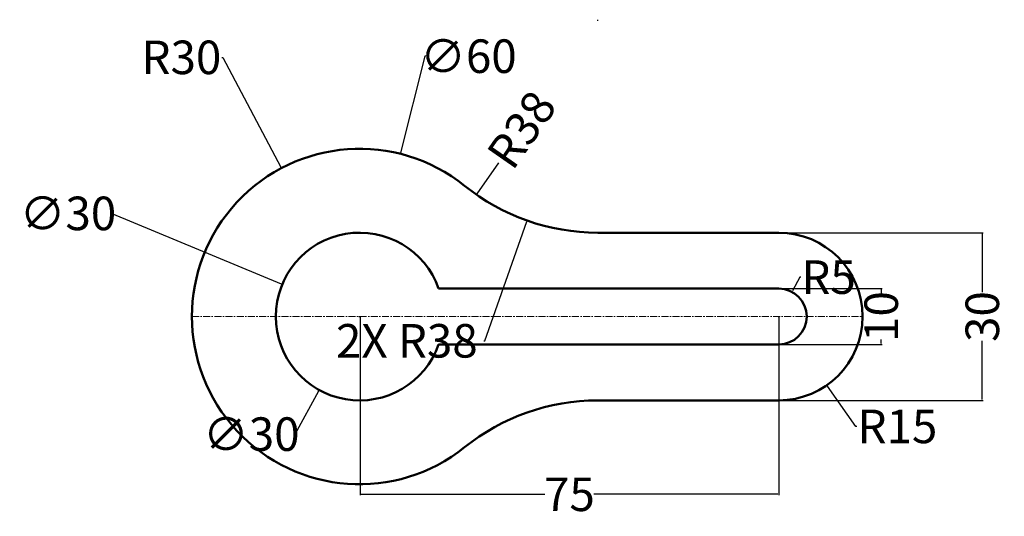
# Model space of a CAD drawing. Units: millimetres. Extents: x 2 to 178, y 21 to 110.
import ezdxf

# ---------------------------------------------------------------- set-up
doc = ezdxf.new("R2010")
doc.units = ezdxf.units.MM
doc.header["$MEASUREMENT"] = 0
doc.linetypes.add('CENTER', pattern=[2, 1.25, -0.25, 0.25, -0.25])
for name, color, linetype, lineweight in [('M-CNTR', 4, 'CENTER', 18), ('M-DIMS', 2, 'Continuous', 25), ('M-OUTL', 7, 'Continuous', 50)]:
    doc.layers.add(name, color=color, linetype=linetype, lineweight=lineweight)
doc.styles.get("Standard").update_dxf_attribs({"font": 'arial.ttf'})
doc.dimstyles.get("Standard").update_dxf_attribs({"dimtxt": 6, "dimasz": 0.18, "dimexe": 0.18, "dimexo": 0.0625, "dimgap": 0.09, "dimtad": 0, "dimtoh": 1, "dimdec": 0, "dimzin": 0, "dimdsep": 46, "dimtxsty": 'Standard', "dimcen": 0.09, "dimadec": 0, "dimazin": 0, "dimtfac": 1, "dimtdec": 0, "dimtofl": 0, "dimtmove": 0, "dimatfit": 3, "dimfxl": 1, "dimtolj": 1, "dimtzin": 0, "dimarcsym": 0})

# ---------------------------------------------------------------- blocks, each defined once
blk = doc.blocks.new('*D1')
at = {"layer": 'Defpoints', "color": 0, "transparency": 16777216}
for p in [(48.73, 83.47), (62.73, 56.94)]:
    blk.add_point(p, dxfattribs=at)
at = {"layer": 'M-DIMS', "color": 0, "lineweight": -2, "transparency": 16777216}
for p, q in [((38.08, 103.3), (38.26, 103.3)), ((38.26, 103.3), (48.64, 83.63)), ((62.64, 56.94), (62.82, 56.94)), ((62.73, 56.85), (62.73, 57.03))]:
    blk.add_line(p, q, dxfattribs=at)
at = {"layer": 'M-DIMS', "color": 0, "transparency": 16777216}
blk.add_solid([(48.67, 83.65), (48.61, 83.62), (48.73, 83.47)], dxfattribs=at)
at = {"layer": 'M-DIMS', "color": 0, "transparency": 16777216, "insert": (30.83, 103.3), "char_height": 6, "attachment_point": 5}
blk.add_mtext('\\A1;R30', dxfattribs=at)
blk = doc.blocks.new('*D2')
at = {"layer": 'Defpoints', "color": 0, "transparency": 16777216}
for p in [(105.33, 109.94), (83.61, 78.76)]:
    blk.add_point(p, dxfattribs=at)
at = {"layer": 'M-DIMS', "color": 0, "lineweight": -2, "transparency": 16777216}
blk.add_line((87.56, 84.43), (83.71, 78.91), dxfattribs=at)
at = {"layer": 'M-DIMS', "color": 0, "transparency": 16777216}
blk.add_solid([(83.69, 78.93), (83.74, 78.89), (83.61, 78.76)], dxfattribs=at)
at = {"layer": 'M-DIMS', "color": 0, "transparency": 16777216, "insert": (91.71, 90.39), "char_height": 6, "attachment_point": 5, "rotation": 55.1393}
blk.add_mtext('\\A1;R38', dxfattribs=at)
blk = doc.blocks.new('*D3')
at = {"layer": 'Defpoints', "color": 0, "transparency": 16777216}
for p in [(62.82, 56.94), (137.73, 56.94), (137.73, 25.15)]:
    blk.add_point(p, dxfattribs=at)
at = {"layer": 'M-DIMS', "color": 0, "lineweight": -2, "transparency": 16777216}
for p, q in [((62.82, 56.88), (62.82, 24.97)), ((137.73, 56.88), (137.73, 24.97)), ((63, 25.15), (95.89, 25.15)), ((137.55, 25.15), (104.66, 25.15))]:
    blk.add_line(p, q, dxfattribs=at)
at = {"layer": 'M-DIMS', "color": 0, "transparency": 16777216}
for points in [[(63, 25.18), (63, 25.12), (62.82, 25.15)], [(137.55, 25.18), (137.55, 25.12), (137.73, 25.15)]]:
    blk.add_solid(points, dxfattribs=at)
at = {"layer": 'M-DIMS', "color": 0, "transparency": 16777216, "insert": (100.27, 25.15), "char_height": 6, "attachment_point": 5}
blk.add_mtext('\\A1;75', dxfattribs=at)
blk = doc.blocks.new('*D4')
at = {"layer": 'Defpoints', "color": 0, "transparency": 16777216}
for p in [(137.73, 71.94), (137.73, 41.94), (174.16, 41.94)]:
    blk.add_point(p, dxfattribs=at)
at = {"layer": 'M-DIMS', "color": 0, "lineweight": -2, "transparency": 16777216}
for p, q in [((137.79, 71.94), (174.34, 71.94)), ((174.16, 71.76), (174.16, 61.32)), ((174.16, 42.12), (174.16, 52.57)), ((137.79, 41.94), (174.34, 41.94))]:
    blk.add_line(p, q, dxfattribs=at)
at = {"layer": 'M-DIMS', "color": 0, "transparency": 16777216}
for points in [[(174.13, 71.76), (174.19, 71.76), (174.16, 71.94)], [(174.13, 42.12), (174.19, 42.12), (174.16, 41.94)]]:
    blk.add_solid(points, dxfattribs=at)
at = {"layer": 'M-DIMS', "color": 0, "transparency": 16777216, "insert": (174.16, 56.94), "char_height": 6, "attachment_point": 5, "rotation": 90}
blk.add_mtext('\\A1;30', dxfattribs=at)
blk = doc.blocks.new('*D5')
at = {"layer": 'Defpoints', "color": 0, "transparency": 16777216}
for p in [(137.73, 61.94), (137.73, 51.94), (156.07, 51.94)]:
    blk.add_point(p, dxfattribs=at)
at = {"layer": 'M-DIMS', "color": 0, "lineweight": -2, "transparency": 16777216}
for p, q in [((137.79, 61.94), (156.25, 61.94)), ((156.07, 61.76), (156.07, 61.04)), ((137.79, 51.94), (156.25, 51.94)), ((156.07, 52.12), (156.07, 52.85))]:
    blk.add_line(p, q, dxfattribs=at)
at = {"layer": 'M-DIMS', "color": 0, "transparency": 16777216}
for points in [[(156.04, 61.76), (156.1, 61.76), (156.07, 61.94)], [(156.04, 52.12), (156.1, 52.12), (156.07, 51.94)]]:
    blk.add_solid(points, dxfattribs=at)
at = {"layer": 'M-DIMS', "color": 0, "transparency": 16777216, "insert": (156.07, 56.94), "char_height": 6, "attachment_point": 5, "rotation": 90}
blk.add_mtext('\\A1;10', dxfattribs=at)
blk = doc.blocks.new('*D6')
at = {"layer": 'Defpoints', "color": 0, "transparency": 16777216}
for p in [(48.88, 62.7), (76.58, 51.19)]:
    blk.add_point(p, dxfattribs=at)
at = {"layer": 'M-DIMS', "color": 0, "lineweight": -2, "transparency": 16777216}
for p, q in [((18.17, 75.39), (18.35, 75.39)), ((18.35, 75.39), (48.71, 62.77)), ((62.64, 56.94), (62.82, 56.94)), ((62.73, 56.85), (62.73, 57.03))]:
    blk.add_line(p, q, dxfattribs=at)
at = {"layer": 'M-DIMS', "color": 0, "transparency": 16777216}
blk.add_solid([(48.72, 62.8), (48.7, 62.74), (48.88, 62.7)], dxfattribs=at)
at = {"layer": 'M-DIMS', "color": 0, "transparency": 16777216, "insert": (10.53, 75.39), "char_height": 6, "attachment_point": 5}
blk.add_mtext('\\A1;∅30', dxfattribs=at)
blk = doc.blocks.new('*D7')
at = {"layer": 'Defpoints', "color": 0, "transparency": 16777216}
for p in [(70.01, 86.05), (55.45, 27.84)]:
    blk.add_point(p, dxfattribs=at)
at = {"layer": 'M-DIMS', "color": 0, "lineweight": -2, "transparency": 16777216}
for p, q in [((74.38, 103.51), (70.06, 86.22)), ((74.56, 103.51), (74.38, 103.51)), ((62.64, 56.94), (62.82, 56.94)), ((62.73, 56.85), (62.73, 57.03))]:
    blk.add_line(p, q, dxfattribs=at)
at = {"layer": 'M-DIMS', "color": 0, "transparency": 16777216}
blk.add_solid([(70.03, 86.23), (70.08, 86.21), (70.01, 86.05)], dxfattribs=at)
at = {"layer": 'M-DIMS', "color": 0, "transparency": 16777216, "insert": (82.2, 103.51), "char_height": 6, "attachment_point": 5}
blk.add_mtext('\\A1;∅60', dxfattribs=at)
blk = doc.blocks.new('*D8')
at = {"layer": 'Defpoints', "color": 0, "transparency": 16777216}
for p in [(69.96, 70.09), (55.5, 43.8)]:
    blk.add_point(p, dxfattribs=at)
at = {"layer": 'M-DIMS', "color": 0, "lineweight": -2, "transparency": 16777216}
for p, q in [((62.64, 56.94), (62.82, 56.94)), ((62.73, 56.85), (62.73, 57.03)), ((51.16, 35.91), (55.41, 43.64)), ((50.98, 35.91), (51.16, 35.91))]:
    blk.add_line(p, q, dxfattribs=at)
at = {"layer": 'M-DIMS', "color": 0, "transparency": 16777216}
blk.add_solid([(55.39, 43.66), (55.44, 43.63), (55.5, 43.8)], dxfattribs=at)
at = {"layer": 'M-DIMS', "color": 0, "transparency": 16777216, "insert": (43.34, 35.91), "char_height": 6, "attachment_point": 5}
blk.add_mtext('\\A1;∅30', dxfattribs=at)
blk = doc.blocks.new('*D9')
at = {"layer": 'Defpoints', "color": 0, "transparency": 16777216}
for p in [(105.33, 109.94), (92.7, 74.1)]:
    blk.add_point(p, dxfattribs=at)
at = {"layer": 'M-DIMS', "color": 0, "lineweight": -2, "transparency": 16777216}
for p, q in [((105.24, 109.94), (105.42, 109.94)), ((105.33, 109.85), (105.33, 110.03)), ((85.12, 52.6), (92.64, 73.93)), ((84.94, 52.6), (85.12, 52.6))]:
    blk.add_line(p, q, dxfattribs=at)
at = {"layer": 'M-DIMS', "color": 0, "transparency": 16777216}
blk.add_solid([(92.61, 73.94), (92.67, 73.92), (92.7, 74.1)], dxfattribs=at)
at = {"layer": 'M-DIMS', "color": 0, "transparency": 16777216, "insert": (71.18, 52.6), "char_height": 6, "attachment_point": 5}
blk.add_mtext('\\A1;2X R38', dxfattribs=at)
blk = doc.blocks.new('*D10')
at = {"layer": 'Defpoints', "color": 0, "transparency": 16777216}
for p in [(137.73, 56.94), (146.34, 44.66)]:
    blk.add_point(p, dxfattribs=at)
at = {"layer": 'M-DIMS', "color": 0, "lineweight": -2, "transparency": 16777216}
for p, q in [((137.64, 56.94), (137.82, 56.94)), ((137.73, 56.85), (137.73, 57.03)), ((151.51, 37.29), (146.44, 44.51)), ((151.69, 37.29), (151.51, 37.29))]:
    blk.add_line(p, q, dxfattribs=at)
at = {"layer": 'M-DIMS', "color": 0, "transparency": 16777216}
blk.add_solid([(146.47, 44.53), (146.42, 44.5), (146.34, 44.66)], dxfattribs=at)
at = {"layer": 'M-DIMS', "color": 0, "transparency": 16777216, "insert": (158.97, 37.29), "char_height": 6, "attachment_point": 5}
blk.add_mtext('\\A1;R15', dxfattribs=at)
blk = doc.blocks.new('*D11')
at = {"layer": 'Defpoints', "color": 0, "transparency": 16777216}
for p in [(140.1, 61.35), (137.73, 56.94)]:
    blk.add_point(p, dxfattribs=at)
at = {"layer": 'M-DIMS', "color": 0, "lineweight": -2, "transparency": 16777216}
for p, q in [((141.52, 63.99), (140.18, 61.51)), ((141.7, 63.99), (141.52, 63.99)), ((137.64, 56.94), (137.82, 56.94)), ((137.73, 56.85), (137.73, 57.03))]:
    blk.add_line(p, q, dxfattribs=at)
at = {"layer": 'M-DIMS', "color": 0, "transparency": 16777216}
blk.add_solid([(140.16, 61.52), (140.21, 61.49), (140.1, 61.35)], dxfattribs=at)
at = {"layer": 'M-DIMS', "color": 0, "transparency": 16777216, "insert": (146.65, 63.99), "char_height": 6, "attachment_point": 5}
blk.add_mtext('\\A1;R5', dxfattribs=at)

msp = doc.modelspace()

# ---------------------------------------------------------------- linework, layer by layer
at = {"layer": 'M-CNTR'}
msp.add_line((32.73, 56.94), (152.73, 56.94), dxfattribs=at)
at = {"layer": 'M-OUTL'}
for points in [[(81.52, 80.33, 0.170903), (105.33, 71.94), (137.73, 71.94, -1), (137.73, 41.94), (105.33, 41.94, 0.170903), (81.52, 33.56, -2.086846)], [(76.87, 61.94), (137.73, 61.94, -1), (137.73, 51.94), (76.87, 51.94, -5.828427)]]:
    msp.add_lwpolyline(points, format="xyb", close=True, dxfattribs=at)

# ---------------------------------------------------------------- dimensions: what is measured, and where the dimension line sits
at = {"layer": 'M-DIMS'}
dim = msp.add_radius_dim(center=(105.33, 109.94), mpoint=(92.7, 74.1), text='2X <>', dimstyle='Standard', override={"dimdec": 0, "dimlfac": 1, "dimrnd": 0, "dimzin": 0, "dimdsep": 46, "dimlunit": 2}, dxfattribs=at)
dim.commit()
dim.dimension.update_dxf_attribs({"geometry": '*D9', "text_midpoint": (71.18, 52.6), "dimtype": 164})
for center, mpoint, override, picture, middle in [((105.33, 109.94), (83.61, 78.76), {"dimclrd": 0, "dimclre": 0, "dimclrt": 0}, '*D2', (91.71, 90.39)), ((62.73, 56.94), (48.73, 83.47), {"dimclrd": 0, "dimclre": 0, "dimclrt": 0}, '*D1', (30.83, 103.3)), ((137.73, 56.94), (140.1, 61.35), {"dimdec": 0, "dimlfac": 1, "dimrnd": 0, "dimzin": 0, "dimdsep": 46, "dimlunit": 2}, '*D11', (146.65, 63.99)), ((137.73, 56.94), (146.34, 44.66), {"dimdec": 0, "dimlfac": 1, "dimrnd": 0, "dimzin": 0, "dimdsep": 46, "dimlunit": 2}, '*D10', (158.97, 37.29))]:
    dim = msp.add_radius_dim(center=center, mpoint=mpoint, dimstyle='Standard', override=override, dxfattribs=at)
    dim.commit()
    dim.dimension.update_dxf_attribs({"geometry": picture, "text_midpoint": middle, "dimtype": 164})
for p1, p2, override, picture, middle in [((55.45, 27.84), (70.01, 86.05), {"dimdec": 0, "dimlfac": 1, "dimrnd": 0, "dimzin": 0, "dimdsep": 46, "dimlunit": 2}, '*D7', (82.2, 103.51)), ((76.58, 51.19), (48.88, 62.7), {"dimclrd": 0, "dimclre": 0, "dimclrt": 0}, '*D6', (10.53, 75.39)), ((69.96, 70.09), (55.5, 43.8), {"dimdec": 0, "dimlfac": 1, "dimrnd": 0, "dimzin": 0, "dimdsep": 46, "dimlunit": 2}, '*D8', (43.34, 35.91))]:
    dim = msp.add_diameter_dim_2p(p1=p1, p2=p2, dimstyle='Standard', override=override, dxfattribs=at)
    dim.commit()
    dim.dimension.update_dxf_attribs({"geometry": picture, "text_midpoint": middle, "dimtype": 163})
for base, p1, p2, picture, middle in [((174.16, 41.94), (137.73, 71.94), (137.73, 41.94), '*D4', (174.16, 56.94)), ((156.07, 51.94), (137.73, 61.94), (137.73, 51.94), '*D5', (156.07, 56.94))]:
    dim = msp.add_linear_dim(base=base, p1=p1, p2=p2, angle=90, dimstyle='Standard', override={"dimclrd": 0, "dimclre": 0, "dimclrt": 0}, dxfattribs=at)
    dim.commit()
    dim.dimension.update_dxf_attribs({"geometry": picture, "text_midpoint": middle})
dim = msp.add_linear_dim(base=(137.73, 25.15), p1=(62.82, 56.94), p2=(137.73, 56.94), dimstyle='Standard', override={"dimclrd": 0, "dimclre": 0, "dimclrt": 0}, dxfattribs=at)
dim.commit()
dim.dimension.update_dxf_attribs({"geometry": '*D3', "text_midpoint": (100.27, 25.15)})

doc.saveas('drawing.dxf')
